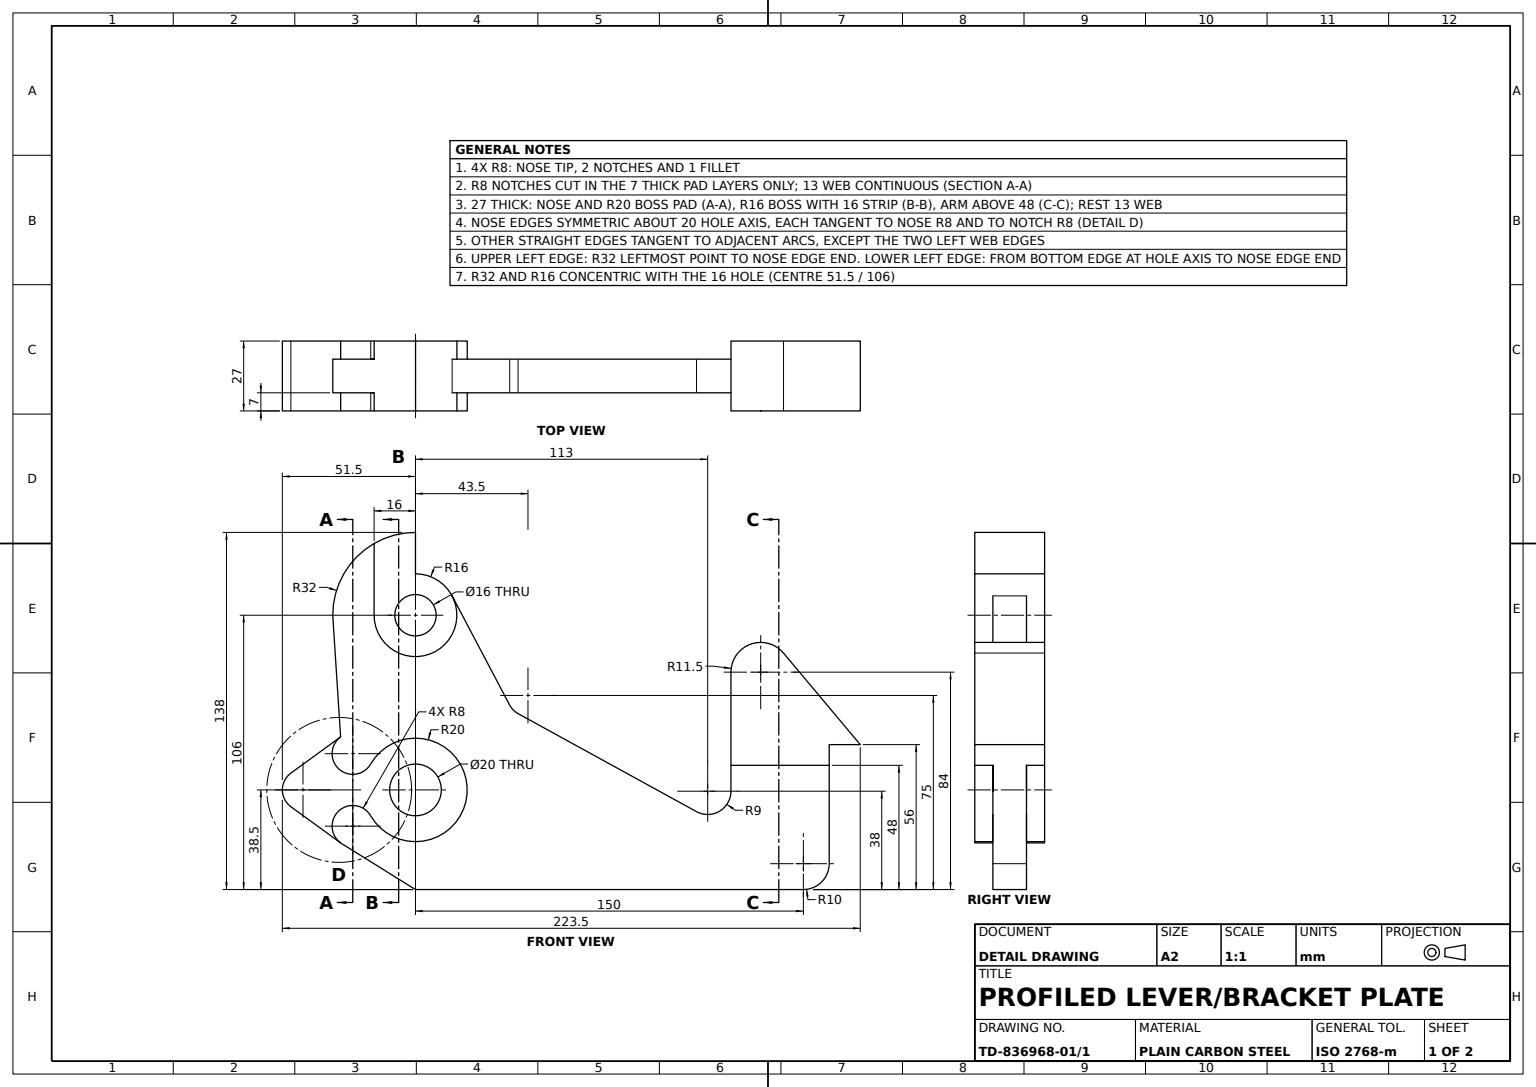
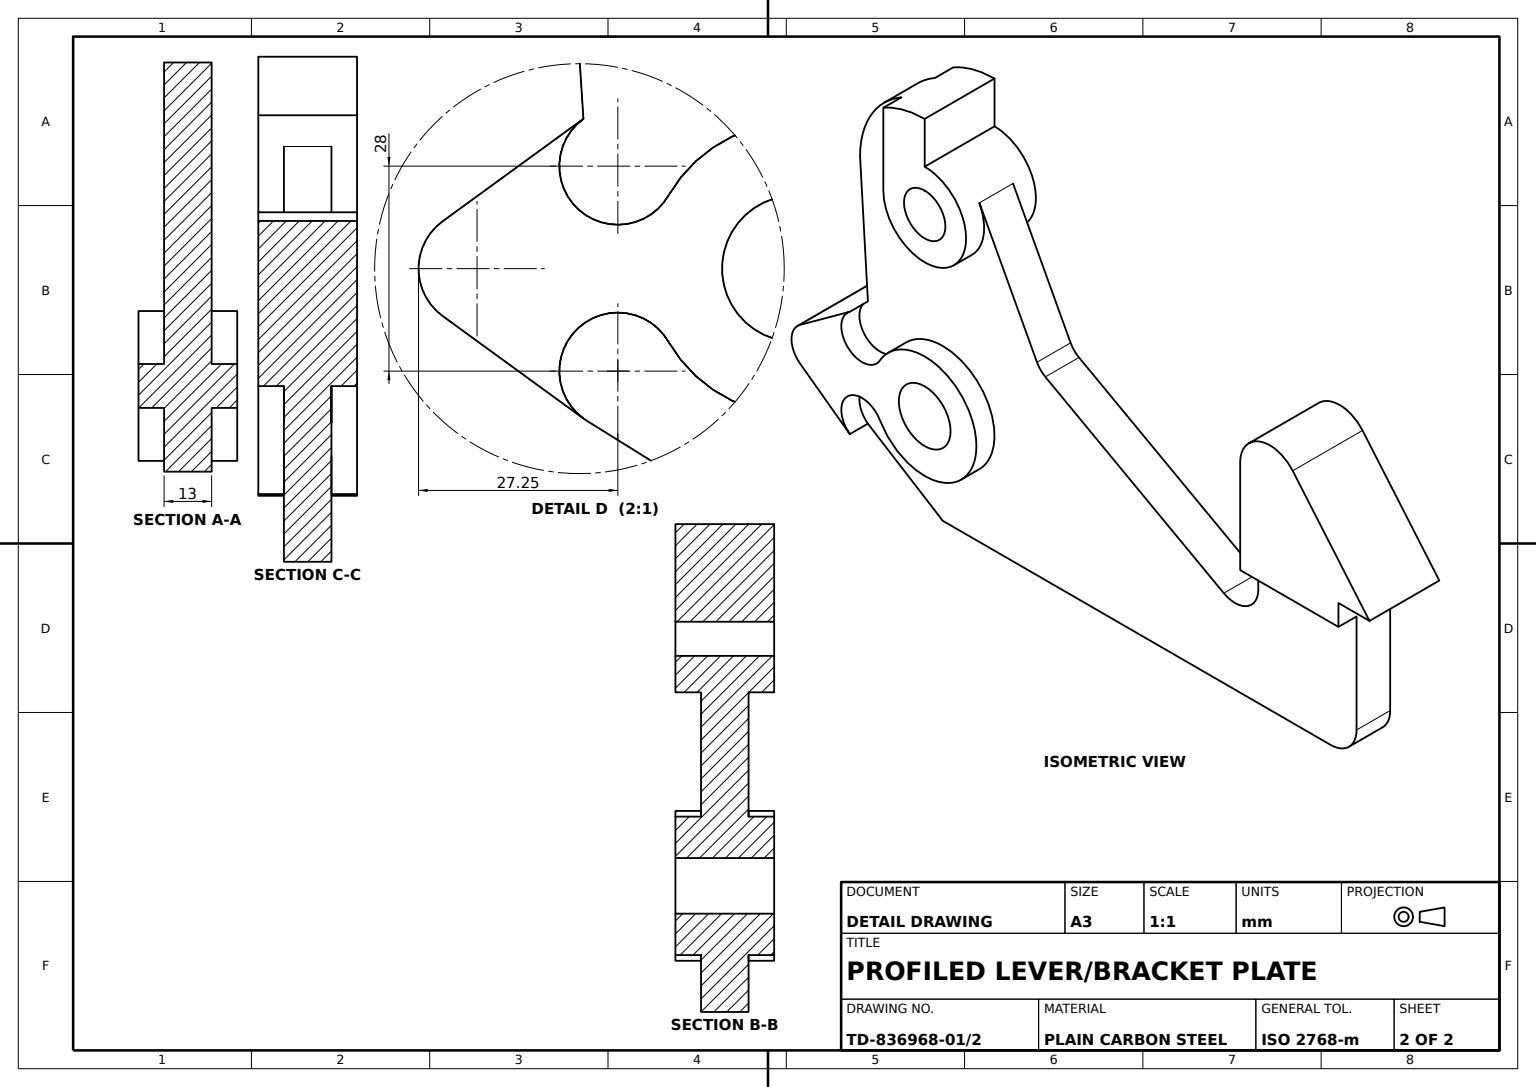
from build123d import *

# Parameters (mm, degrees)
LEVER_PLATE_PROFILE_R   = 10
LEVER_PLATE_PROFILE_R_2 = 8
LEVER_PLATE_DEPTH       = 13
PIVOT_BOSS_PROFILE_R    = 8
PIVOT_BOSS_PROFILE_R_2  = 10
PIVOT_BOSSES_DEPTH      = 13.5


with BuildPart() as part:
    # Lever Plate Profile → Lever Plate (new body)
    with BuildSketch(Plane(origin=(0, 0, 0), x_dir=(1, 0, 0), z_dir=(0, 1, 0))):
        with BuildLine():
            Line((-150, -10), (0, -10))
            ThreePointArc((0, -10), (7.071067812, -7.071067812), (10, 0))
            Line((10, 0), (10, 46))
            Line((10, 46), (22, 46))
            Line((22, 46), (-7.689634159, 81.391038746))
            ThreePointArc((-7.689634159, 81.391038746), (-20.432606822, 84.806692537), (-28, 74))
            Line((-28, 74), (-28, 28))
            ThreePointArc((-28, 28), (-32.415747822, 20.255025373), (-41.329918215, 20.110018488))
            Line((-41.329918215, 20.110018488), (-110.348816191, 57.986683101))
            ThreePointArc((-110.348816191, 57.986683101), (-112.202667383, 59.389332952), (-113.574982592, 61.265750233))
            Line((-113.574982592, 61.265750233), (-135.850034815, 103.468499533))
            ThreePointArc((-135.850034815, 103.468499533), (-141.738522908, 109.702116489), (-150, 112))
            Line((-150, 112), (-150, 128))
            ThreePointArc((-150, 128), (-172.627416998, 118.627416998), (-182, 96))
            Line((-182, 96), (-178.953878866, 48.970038503))
            Line((-178.953878866, 48.970038503), (-198.20516756, 34.970038503))
            ThreePointArc((-198.20516756, 34.970038503), (-201.5, 28.5), (-198.20516756, 22.029961497))
            Line((-198.20516756, 22.029961497), (-178.953878866, 8.029961497))
            ThreePointArc((-178.953878866, 8.029961497), (-178.716545197, 7.863851996), (-178.473353106, 7.706444107))
            Line((-178.473353106, 7.706444107), (-150, -10))
        make_face()
        with Locations(Location((-150, 28.5, 0), (0, 0, 90))):
            Circle(LEVER_PLATE_PROFILE_R, mode=Mode.SUBTRACT)
        with Locations(Location((-150, 96, 0), (0, 0, 90))):
            Circle(LEVER_PLATE_PROFILE_R_2, mode=Mode.SUBTRACT)
    extrude(amount=LEVER_PLATE_DEPTH)

    # Pivot Boss Profile → Pivot Bosses (add, symmetric)
    # profile 1 of 3: a face of its own
    with BuildSketch(Plane(origin=(0, 6.5, 0), x_dir=(1, 0, 0), z_dir=(0, 1, 0))):
        with BuildLine():
            Line((-150, 112), (-150, 128))
            ThreePointArc((-150, 128), (-158.282209443, 126.909626441), (-166, 123.712812921))
            Line((-166, 123.712812921), (-166, 96))
            ThreePointArc((-166, 96), (-138.686291501, 84.686291501), (-150, 112))
        make_face()
        with Locations(Location((-150, 96, 0), (0, 0, 90))):
            Circle(PIVOT_BOSS_PROFILE_R, mode=Mode.SUBTRACT)
    # profile 2 of 3: a face of its own
    with BuildSketch(Plane(origin=(0, 6.5, 0), x_dir=(1, 0, 0), z_dir=(0, 1, 0))):
        with BuildLine():
            Line((-198.20516756, 34.970038503), (-178.953878866, 48.970038503))
            ThreePointArc((-178.953878866, 48.970038503), (-179.600430512, 36.553648048), (-167.320508076, 38.5))
            ThreePointArc((-167.320508076, 38.5), (-130, 28.5), (-167.320508076, 18.5))
            ThreePointArc((-167.320508076, 18.5), (-179.600430512, 20.446351952), (-178.953878866, 8.029961497))
            Line((-178.953878866, 8.029961497), (-198.20516756, 22.029961497))
            ThreePointArc((-198.20516756, 22.029961497), (-201.5, 28.5), (-198.20516756, 34.970038503))
        make_face()
        with Locations(Location((-150, 28.5, 0), (0, 0, 90))):
            Circle(PIVOT_BOSS_PROFILE_R_2, mode=Mode.SUBTRACT)
    # profile 3 of 3: a face of its own
    with BuildSketch(Plane(origin=(0, 6.5, 0), x_dir=(1, 0, 0), z_dir=(0, 1, 0))):
        with BuildLine():
            Line((-7.689634159, 81.391038746), (22, 46))
            Line((22, 46), (10, 46))
            Line((10, 46), (10, 38))
            Line((10, 38), (-28, 38))
            Line((-28, 38), (-28, 74))
            ThreePointArc((-28, 74), (-20.432606822, 84.806692537), (-7.689634159, 81.391038746))
        make_face()
    extrude(amount=PIVOT_BOSSES_DEPTH, both=True)


solid = part.part
